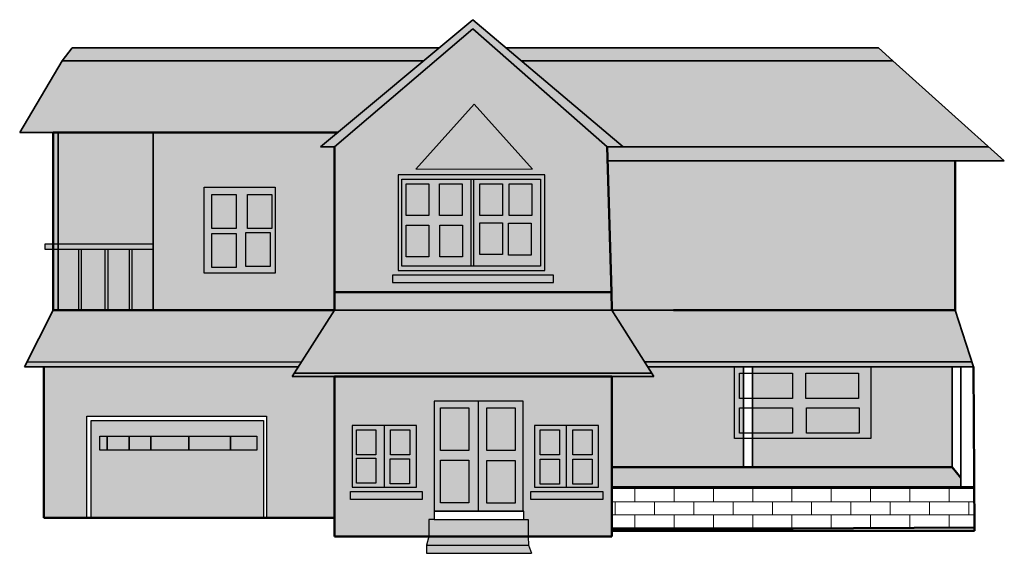
# Model space of a CAD drawing. Units: millimetres. Extents: x 69 to 5162, y 1088 to 3851.
import ezdxf

# ---------------------------------------------------------------- set-up
doc = ezdxf.new("R2010")
doc.units = ezdxf.units.MM
for name, color, linetype, lineweight in [('A-COLS', 7, 'Continuous', 35), ('A-DETL', 7, 'Continuous', 18), ('A-DOOR', 3, 'Continuous', 25), ('A-ELEV-PATT', 252, 'Continuous', 13), ('A-FLOR-HRAL', 6, 'Continuous', 25), ('A-FLOR-STRS', 3, 'Continuous', 25), ('A-GLAZ', 4, 'Continuous', 25), ('A-ROOF', 30, 'Continuous', 35), ('A-WALL', 7, 'Continuous', 50), ('A-WALL-PATT', 8, 'Continuous', 13)]:
    doc.layers.add(name, color=color, linetype=linetype, lineweight=lineweight)

msp = doc.modelspace()

# ---------------------------------------------------------------- hatches: boundary and pattern name
at = {"layer": 'A-ELEV-PATT'}
h = msp.add_hatch(color=256, dxfattribs=at)
h.set_gradient(color1=(169, 83, 160), color2=(169, 83, 160))
h.paths.add_polyline_path([(511.8, 2661), (389.1, 2661), (389.1, 2346.9), (511.8, 2346.9)])
h.paths.add_polyline_path([(636.7, 2661), (527.2, 2661), (527.2, 2346.9), (636.7, 2346.9)])
h.paths.add_polyline_path([(759.8, 2661), (651, 2661), (651, 2346.9), (759.8, 2346.9)])
h.paths.add_polyline_path([(374.7, 2661), (267.5, 2661), (267.5, 2346.9), (374.7, 2346.9)])
h.paths.add_polyline_path([(4892.2, 1533.1), (3131.8, 1533.1), (3131.8, 1431.2), (4937.5, 1431.2), (4937.5, 1478.9)])
h.paths.add_polyline_path([(944.6, 1695.1), (747.8, 1695.1), (747.8, 1621.5), (944.6, 1621.5)])
h.paths.add_polyline_path([(1159.7, 1695.1), (944.6, 1695.1), (944.6, 1621.5), (1159.7, 1621.5)])
h.paths.add_polyline_path([(1295.8, 1695.1), (1159.7, 1695.1), (1159.7, 1621.5), (1295.8, 1621.5)])
h.paths.add_polyline_path([(636.1, 1695.1), (521.5, 1695.1), (521.5, 1621.5), (636.1, 1621.5)])
h.paths.add_polyline_path([(747.8, 1695.1), (636.1, 1695.1), (636.1, 1621.5), (747.8, 1621.5)])
h.paths.add_polyline_path([(521.5, 1695.1), (482.9, 1695.1), (482.9, 1621.5), (521.5, 1621.5)])
h.paths.add_polyline_path([(2829.8, 2527.8), (1997.6, 2527.8), (1997.6, 2490.3), (2829.8, 2490.3)])
h.paths.add_polyline_path([(2786.1, 3048.5), (2027.1, 3048.5), (2027.1, 2552.8), (2786.1, 2552.8)])
h.paths.add_polyline_path([(2045.2, 2575.6), (2045.2, 3025.8), (2762.5, 3025.8), (2762.5, 2575.6)], flags=16)
h.paths.add_polyline_path([(2242.5, 2623.4), (2242.5, 2787.9), (2359.8, 2787.9), (2359.8, 2623.4)], flags=0)
h.paths.add_polyline_path([(2449.3, 2634.7), (2449.3, 2799.2), (2566.6, 2799.2), (2566.6, 2634.7)], flags=0)
h.paths.add_polyline_path([(2186, 2623.4), (2068.8, 2623.4), (2068.8, 2787.9), (2186, 2787.9)], flags=0)
h.paths.add_polyline_path([(2240.2, 2837.1), (2240.2, 3001.6), (2357.5, 3001.6), (2357.5, 2837.1)], flags=0)
h.paths.add_polyline_path([(2597.1, 2632.5), (2597.1, 2797), (2714.3, 2797), (2714.3, 2632.5)], flags=0)
h.paths.add_polyline_path([(2449.3, 2837.1), (2449.3, 3001.6), (2566.6, 3001.6), (2566.6, 2837.1)], flags=0)
h.paths.add_polyline_path([(2186, 2837.1), (2068.8, 2837.1), (2068.8, 3001.6), (2186, 3001.6)], flags=0)
h.paths.add_polyline_path([(2601.6, 2837.1), (2601.6, 3001.6), (2718.9, 3001.6), (2718.9, 2837.1)], flags=0)
h.paths.add_polyline_path([(1390.1, 2983.9), (1023.5, 2983.9), (1023.5, 2539.3), (1390.1, 2539.3)])
h.paths.add_polyline_path([(1239.1, 2749.6), (1365.2, 2749.6), (1365.2, 2573.5), (1239.1, 2573.5)], flags=16)
h.paths.add_polyline_path([(1189, 2568.7), (1062.9, 2568.7), (1062.9, 2744.7), (1189, 2744.7)], flags=16)
h.paths.add_polyline_path([(1247.2, 2769), (1247.2, 2945.1), (1373.3, 2945.1), (1373.3, 2769)], flags=16)
h.paths.add_polyline_path([(1189, 2769), (1062.9, 2769), (1062.9, 2945.1), (1189, 2945.1)], flags=16)
h.paths.add_polyline_path([(4471.7, 2052.7), (3859.7, 2052.7), (3859.7, 2020.4), (4066.3, 2020.4), (4066.3, 1889), (3859.7, 1889), (3859.7, 1841.9), (4066.3, 1841.9), (4066.3, 1710.5), (3859.7, 1710.5), (3859.7, 1683), (4471.7, 1683)])
h.paths.add_polyline_path([(4135.3, 1889), (4135.3, 2020.4), (4408.2, 2020.4), (4408.2, 1889)], flags=16)
h.paths.add_polyline_path([(4138.6, 1841.9), (4411.5, 1841.9), (4411.5, 1710.5), (4138.6, 1710.5)], flags=16)
h.paths.add_polyline_path([(3793.4, 1841.9), (3813.9, 1841.9), (3813.9, 1889), (3793.4, 1889), (3793.4, 2020.4), (3813.9, 2020.4), (3813.9, 2052.7), (3766.7, 2052.7), (3766.7, 1683), (3813.9, 1683), (3813.9, 1710.5), (3793.4, 1710.5)])
h.paths.add_polyline_path([(2442.6, 1875.6), (2212.5, 1875.6), (2212.5, 1306.4), (2442.6, 1306.4)])
h.paths.add_polyline_path([(2392.3, 1620), (2245.7, 1620), (2245.7, 1841.2), (2392.3, 1841.2)], flags=16)
h.paths.add_polyline_path([(2392.3, 1570.2), (2392.3, 1348.9), (2245.7, 1348.9), (2245.7, 1570.2)], flags=16)
h.paths.add_polyline_path([(2672.8, 1875.6), (2442.6, 1875.6), (2442.6, 1306.4), (2672.8, 1306.4)])
h.paths.add_polyline_path([(2486.1, 1620), (2486.1, 1841.2), (2632.7, 1841.2), (2632.7, 1620)], flags=16)
h.paths.add_polyline_path([(2486.1, 1568.7), (2632.7, 1568.7), (2632.7, 1347.5), (2486.1, 1347.5)], flags=16)
h.paths.add_polyline_path([(1955.6, 1749.4), (1789.6, 1749.4), (1789.6, 1431), (1955.6, 1431)])
h.paths.add_polyline_path([(1911.6, 1451.2), (1811.8, 1451.2), (1811.8, 1580.1), (1911.6, 1580.1)], flags=16)
h.paths.add_polyline_path([(1911.6, 1597.9), (1811.8, 1597.9), (1811.8, 1726.8), (1911.6, 1726.8)], flags=16)
h.paths.add_polyline_path([(2121.7, 1749.4), (1955.6, 1749.4), (1955.6, 1431), (2121.7, 1431)])
h.paths.add_polyline_path([(1986, 1577.2), (2085.8, 1577.2), (2085.8, 1448.3), (1986, 1448.3)], flags=16)
h.paths.add_polyline_path([(1986.9, 1597.9), (1986.9, 1726.8), (2086.7, 1726.8), (2086.7, 1597.9)], flags=16)
h.paths.add_polyline_path([(2151.4, 1408), (1779.5, 1408), (1779.5, 1367.3), (2151.4, 1367.3)])
h.paths.add_polyline_path([(3085.7, 1408), (2713.8, 1408), (2713.8, 1367.3), (3085.7, 1367.3)])
h.paths.add_polyline_path([(2897.4, 1749.4), (2731.3, 1749.4), (2731.3, 1431), (2897.4, 1431)])
h.paths.add_polyline_path([(2860.7, 1446.6), (2760.9, 1446.6), (2760.9, 1575.5), (2860.7, 1575.5)], flags=16)
h.paths.add_polyline_path([(2860.7, 1597.9), (2760.9, 1597.9), (2760.9, 1726.8), (2860.7, 1726.8)], flags=16)
h.paths.add_polyline_path([(3063.5, 1749.4), (2897.4, 1749.4), (2897.4, 1431), (3063.5, 1431)])
h.paths.add_polyline_path([(2929.9, 1575.5), (3029.7, 1575.5), (3029.7, 1446.6), (2929.9, 1446.6)], flags=16)
h.paths.add_polyline_path([(2929.9, 1597.9), (2929.9, 1726.8), (3029.7, 1726.8), (3029.7, 1597.9)], flags=16)
h.paths.add_polyline_path([(2238.2, 3704.6), (340.3, 3704.6), (288.6, 3637.4), (2157.7, 3637.4)])
h.paths.add_polyline_path([(4510.8, 3704.6), (2586.9, 3704.6), (2666.3, 3637.4), (4585.6, 3637.4)])
h.paths.add_polyline_path([(5080.6, 3193.1), (3107.7, 3193.1), (3109.9, 3119.6), (5162.5, 3119.6)])
h.paths.add_polyline_path([(2413.6, 3851.2), (1625.7, 3193.1), (1697.3, 3193.1), (2413.6, 3803.4), (3023.6, 3267.2), (3107.7, 3193.1), (3191.6, 3193.1)])
h.paths.add_polyline_path([(3129.9, 2440.9), (1697.3, 2440.9), (1697.3, 2346.9), (3131.8, 2346.9)])
h = msp.add_hatch(color=256, dxfattribs=at)
h.set_gradient(color1=(122, 175, 223), color2=(122, 175, 223))
h.paths.add_polyline_path([(1697.3, 3193.1), (1625.7, 3193.1), (1714.3, 3267.2), (759.8, 3267.2), (759.8, 2346.9), (1697.3, 2346.9), (1697.3, 2440.9)])
h.paths.add_polyline_path([(1023.5, 2983.9), (1390.1, 2983.9), (1390.1, 2539.3), (1023.5, 2539.3)], flags=16)
h.paths.add_polyline_path([(1062.9, 2945.1), (1189, 2945.1), (1189, 2769), (1062.9, 2769)], flags=0)
h.paths.add_polyline_path([(1062.9, 2744.7), (1189, 2744.7), (1189, 2568.7), (1062.9, 2568.7)], flags=0)
h.paths.add_polyline_path([(1247.2, 2945.1), (1373.3, 2945.1), (1373.3, 2769), (1247.2, 2769)], flags=0)
h.paths.add_polyline_path([(1239.1, 2749.6), (1365.2, 2749.6), (1365.2, 2573.5), (1239.1, 2573.5)], flags=0)
h.paths.add_polyline_path([(4907.8, 3119.6), (3109.9, 3119.6), (3129.9, 2440.9), (3131.8, 2346.9), (3452, 2346.9), (4907.8, 2346.9)])
h.paths.add_polyline_path([(3109.9, 3119.6), (3107.7, 3193.1), (3023.6, 3267.2), (2413.6, 3803.4), (1697.3, 3193.1), (1697.3, 2440.9), (3129.9, 2440.9)])
h.paths.add_polyline_path([(2786.1, 2552.8), (2027.1, 2552.8), (2027.1, 3048.5), (2786.1, 3048.5)], flags=16)
h.paths.add_polyline_path([(2762.5, 2575.6), (2045.2, 2575.6), (2045.2, 3025.8), (2762.5, 3025.8)], flags=0)
h.paths.add_polyline_path([(2718.9, 2837.1), (2601.6, 2837.1), (2601.6, 3001.6), (2718.9, 3001.6)], flags=0)
h.paths.add_polyline_path([(2714.3, 2797), (2714.3, 2632.5), (2597.1, 2632.5), (2597.1, 2797)], flags=0)
h.paths.add_polyline_path([(2722, 3077.5), (2119, 3077.5), (2420.5, 3413.6)], flags=16)
h.paths.add_polyline_path([(2829.8, 2527.8), (2829.8, 2490.3), (1997.6, 2490.3), (1997.6, 2527.8)], flags=16)
h.paths.add_polyline_path([(2566.6, 2837.1), (2449.3, 2837.1), (2449.3, 3001.6), (2566.6, 3001.6)], flags=0)
h.paths.add_polyline_path([(2566.6, 2799.2), (2566.6, 2634.7), (2449.3, 2634.7), (2449.3, 2799.2)], flags=0)
h.paths.add_polyline_path([(2357.5, 2837.1), (2240.2, 2837.1), (2240.2, 3001.6), (2357.5, 3001.6)], flags=0)
h.paths.add_polyline_path([(2359.8, 2787.9), (2359.8, 2623.4), (2242.5, 2623.4), (2242.5, 2787.9)], flags=0)
h.paths.add_polyline_path([(2186, 2837.1), (2068.8, 2837.1), (2068.8, 3001.6), (2186, 3001.6)], flags=0)
h.paths.add_polyline_path([(2186, 2787.9), (2186, 2623.4), (2068.8, 2623.4), (2068.8, 2787.9)], flags=0)
h.paths.add_polyline_path([(3766.7, 2052.7), (3318.2, 2052.7), (3349.6, 2003.2), (3131.8, 2003.2), (3131.8, 1533.1), (3813.9, 1533.1), (3813.9, 1683), (3766.7, 1683)])
h.paths.add_polyline_path([(4892.2, 2052.7), (4471.7, 2052.7), (4471.7, 1683), (3859.7, 1683), (3859.7, 1533.1), (4892.2, 1533.1)])
h.paths.add_polyline_path([(1697.3, 2003.2), (1478.5, 2003.2), (1510, 2052.7), (194.2, 2052.7), (194.2, 1271.1), (416.8, 1271.1), (416.8, 1797.4), (1345.9, 1797.4), (1345.9, 1271.1), (1697.3, 1271.1)])
h = msp.add_hatch(color=256, dxfattribs=at)
h.set_gradient(color1=(242, 103, 34), color2=(242, 103, 34))
h.paths.add_polyline_path([(2157.7, 3637.4), (288.6, 3637.4), (69, 3267.2), (242.5, 3267.2), (1714.3, 3267.2)])
h.paths.add_polyline_path([(4585.6, 3637.4), (2666.3, 3637.4), (3191.6, 3193.1), (5080.6, 3193.1)])
h.paths.add_polyline_path([(4907.8, 2346.9), (3452, 2346.9), (3131.8, 2346.9), (3300.9, 2080), (4995, 2080)])
h.paths.add_polyline_path([(1697.3, 2346.9), (242.5, 2346.9), (106.8, 2077.5), (1527.5, 2080)])
h.paths.add_polyline_path([(3131.8, 2346.9), (1697.3, 2346.9), (1527.5, 2080), (1489.6, 2020.5), (3338.6, 2020.5)])
h = msp.add_hatch(color=256, dxfattribs=at)
h.set_gradient(color1=(99, 100, 102), color2=(99, 100, 102))
h.paths.add_polyline_path([(759.8, 2690.2), (759.8, 3267.2), (267.5, 3267.2), (267.5, 2690.2)])
h.paths.add_polyline_path([(1330.1, 1271.1), (1330.1, 1775), (439.3, 1775), (439.3, 1271.1)])
h.paths.add_polyline_path([(482.9, 1621.5), (482.9, 1695.1), (1295.8, 1695.1), (1295.8, 1621.5)], flags=16)
h.paths.add_polyline_path([(2119, 3077.5), (2722, 3077.5), (2420.5, 3413.6)])
h.paths.add_polyline_path([(1697.3, 2003.2), (1697.3, 1175.3), (2185.2, 1175.3), (2185.2, 1262.3), (2212.5, 1262.3), (2212.5, 1306.4), (2212.5, 1875.6), (2672.8, 1875.6), (2672.8, 1306.4), (2677.5, 1306.4), (2677.5, 1262.3), (2699, 1262.3), (2699, 1175.3), (3131.8, 1175.3), (3131.8, 2003.2)])
h.paths.add_polyline_path([(3063.5, 1749.4), (3063.5, 1431), (2731.3, 1431), (2731.3, 1749.4)], flags=16)
h.paths.add_polyline_path([(2760.9, 1726.8), (2860.7, 1726.8), (2860.7, 1597.9), (2760.9, 1597.9)], flags=0)
h.paths.add_polyline_path([(2929.9, 1726.8), (3029.7, 1726.8), (3029.7, 1597.9), (2929.9, 1597.9)], flags=0)
h.paths.add_polyline_path([(2760.9, 1575.5), (2860.7, 1575.5), (2860.7, 1446.6), (2760.9, 1446.6)], flags=0)
h.paths.add_polyline_path([(2929.9, 1575.5), (3029.7, 1575.5), (3029.7, 1446.6), (2929.9, 1446.6)], flags=0)
h.paths.add_polyline_path([(3085.7, 1408), (3085.7, 1367.3), (2713.8, 1367.3), (2713.8, 1408)], flags=16)
h.paths.add_polyline_path([(2121.7, 1749.4), (2121.7, 1431), (1789.6, 1431), (1789.6, 1749.4)], flags=16)
h.paths.add_polyline_path([(2086.7, 1726.8), (2086.7, 1597.9), (1986.9, 1597.9), (1986.9, 1726.8)], flags=0)
h.paths.add_polyline_path([(2085.8, 1577.2), (2085.8, 1448.3), (1986, 1448.3), (1986, 1577.2)], flags=0)
h.paths.add_polyline_path([(2151.4, 1408), (2151.4, 1367.3), (1779.5, 1367.3), (1779.5, 1408)], flags=16)
h.paths.add_polyline_path([(1911.6, 1726.8), (1911.6, 1597.9), (1811.8, 1597.9), (1811.8, 1726.8)], flags=0)
h.paths.add_polyline_path([(1911.6, 1580.1), (1911.6, 1451.2), (1811.8, 1451.2), (1811.8, 1580.1)], flags=0)
h = msp.add_hatch(color=256, dxfattribs=at)
h.set_gradient(color1=(255, 255, 255))
h.paths.add_polyline_path([(267.5, 3267.2), (242.5, 3267.2), (242.5, 2690.2), (267.5, 2690.2)])
h.paths.add_polyline_path([(759.8, 2690.2), (267.5, 2690.2), (267.5, 2661), (759.8, 2661)])
h.paths.add_polyline_path([(651, 2661), (636.7, 2661), (636.7, 2346.9), (651, 2346.9)])
h.paths.add_polyline_path([(267.5, 2661), (242.5, 2661), (242.5, 2346.9), (267.5, 2346.9)])
h.paths.add_polyline_path([(267.5, 2690.2), (242.5, 2690.2), (242.5, 2661), (267.5, 2661)])
h.paths.add_polyline_path([(242.5, 2690.2), (200.1, 2690.2), (200.1, 2661), (242.5, 2661)])
h.paths.add_polyline_path([(389.1, 2661), (374.7, 2661), (374.7, 2346.9), (389.1, 2346.9)])
h.paths.add_polyline_path([(527.2, 2661), (511.8, 2661), (511.8, 2346.9), (527.2, 2346.9)])
h.paths.add_polyline_path([(1527.5, 2080), (106.8, 2077.5), (94.3, 2052.7), (1510, 2052.7)])
h.paths.add_polyline_path([(3338.6, 2020.5), (1489.6, 2020.5), (1478.5, 2003.2), (1697.3, 2003.2), (3131.8, 2003.2), (3349.6, 2003.2)])
h.paths.add_polyline_path([(4995, 2080), (3300.9, 2080), (3318.2, 2052.7), (5003.9, 2052.7)])
h = msp.add_hatch(color=256, dxfattribs=at)
h.set_gradient(color1=(0, 255, 255), color2=(0, 255, 255))
h.paths.add_polyline_path([(2068.8, 2837.1), (2186, 2837.1), (2186, 3001.6), (2068.8, 3001.6)])
h.paths.add_polyline_path([(2240.2, 2837.1), (2357.5, 2837.1), (2357.5, 3001.6), (2240.2, 3001.6)])
h.paths.add_polyline_path([(2242.5, 2787.9), (2242.5, 2623.4), (2359.8, 2623.4), (2359.8, 2787.9)])
h.paths.add_polyline_path([(2186, 2787.9), (2068.8, 2787.9), (2068.8, 2623.4), (2186, 2623.4)])
h.paths.add_polyline_path([(2449.3, 2837.1), (2566.6, 2837.1), (2566.6, 3001.6), (2449.3, 3001.6)])
h.paths.add_polyline_path([(2601.6, 2837.1), (2718.9, 2837.1), (2718.9, 3001.6), (2601.6, 3001.6)])
h.paths.add_polyline_path([(2714.3, 2797), (2597.1, 2797), (2597.1, 2632.5), (2714.3, 2632.5)])
h.paths.add_polyline_path([(2449.3, 2634.7), (2566.6, 2634.7), (2566.6, 2799.2), (2449.3, 2799.2)])
h.paths.add_polyline_path([(1247.2, 2769), (1373.3, 2769), (1373.3, 2945.1), (1247.2, 2945.1)])
h.paths.add_polyline_path([(1062.9, 2769), (1189, 2769), (1189, 2945.1), (1062.9, 2945.1)])
h.paths.add_polyline_path([(1062.9, 2568.7), (1189, 2568.7), (1189, 2744.7), (1062.9, 2744.7)])
h.paths.add_polyline_path([(1365.2, 2749.6), (1239.1, 2749.6), (1239.1, 2573.5), (1365.2, 2573.5)])
h.paths.add_polyline_path([(1811.8, 1597.9), (1911.6, 1597.9), (1911.6, 1726.8), (1811.8, 1726.8)])
h.paths.add_polyline_path([(2086.7, 1597.9), (2086.7, 1726.8), (1986.9, 1726.8), (1986.9, 1597.9)])
h.paths.add_polyline_path([(1986, 1448.3), (2085.8, 1448.3), (2085.8, 1577.2), (1986, 1577.2)])
h.paths.add_polyline_path([(1911.6, 1580.1), (1811.8, 1580.1), (1811.8, 1451.2), (1911.6, 1451.2)])
h.paths.add_polyline_path([(2392.3, 1841.2), (2245.7, 1841.2), (2245.7, 1620), (2392.3, 1620)])
h.paths.add_polyline_path([(2860.7, 1597.9), (2860.7, 1726.8), (2760.9, 1726.8), (2760.9, 1597.9)])
h.paths.add_polyline_path([(2860.7, 1575.5), (2760.9, 1575.5), (2760.9, 1446.6), (2860.7, 1446.6)])
h.paths.add_polyline_path([(3029.7, 1726.8), (2929.9, 1726.8), (2929.9, 1597.9), (3029.7, 1597.9)])
h.paths.add_polyline_path([(3029.7, 1575.5), (2929.9, 1575.5), (2929.9, 1446.6), (3029.7, 1446.6)])
h.paths.add_polyline_path([(4066.3, 1889), (4066.3, 2020.4), (3859.7, 2020.4), (3859.7, 1889)])
h.paths.add_polyline_path([(4408.2, 1889), (4408.2, 2020.4), (4135.3, 2020.4), (4135.3, 1889)])
h.paths.add_polyline_path([(4411.5, 1710.5), (4411.5, 1841.9), (4138.6, 1841.9), (4138.6, 1710.5)])
h.paths.add_polyline_path([(4066.3, 1710.5), (4066.3, 1841.9), (3859.7, 1841.9), (3859.7, 1710.5)])
h.paths.add_polyline_path([(3793.4, 1710.5), (3813.9, 1710.5), (3813.9, 1841.9), (3793.4, 1841.9)])
h.paths.add_polyline_path([(3813.9, 2020.4), (3793.4, 2020.4), (3793.4, 1889), (3813.9, 1889)])
h = msp.add_hatch(color=256, dxfattribs=at)
h.set_gradient(color1=(16, 86, 137), color2=(34, 52, 110))
h.paths.add_polyline_path([(2068.8, 2837.1), (2186, 2837.1), (2186, 3001.6), (2068.8, 3001.6)])
h.paths.add_polyline_path([(2240.2, 3001.6), (2240.2, 2837.1), (2357.5, 2837.1), (2357.5, 3001.6)])
h.paths.add_polyline_path([(2449.3, 3001.6), (2449.3, 2837.1), (2566.6, 2837.1), (2566.6, 3001.6)])
h.paths.add_polyline_path([(2601.6, 2837.1), (2718.9, 2837.1), (2718.9, 3001.6), (2601.6, 3001.6)])
h.paths.add_polyline_path([(2597.1, 2632.5), (2714.3, 2632.5), (2714.3, 2797), (2597.1, 2797)])
h.paths.add_polyline_path([(2449.3, 2634.7), (2566.6, 2634.7), (2566.6, 2799.2), (2449.3, 2799.2)])
h.paths.add_polyline_path([(2359.8, 2787.9), (2242.5, 2787.9), (2242.5, 2623.4), (2359.8, 2623.4)])
h.paths.add_polyline_path([(2068.8, 2787.9), (2068.8, 2623.4), (2186, 2623.4), (2186, 2787.9)])
h.paths.add_polyline_path([(1247.2, 2945.1), (1247.2, 2769), (1373.3, 2769), (1373.3, 2945.1)])
h.paths.add_polyline_path([(1365.2, 2749.6), (1239.1, 2749.6), (1239.1, 2573.5), (1365.2, 2573.5)])
h.paths.add_polyline_path([(1189, 2945.1), (1062.9, 2945.1), (1062.9, 2769), (1189, 2769)])
h.paths.add_polyline_path([(1062.9, 2744.7), (1062.9, 2568.7), (1189, 2568.7), (1189, 2744.7)])
h.paths.add_polyline_path([(1911.6, 1726.8), (1811.8, 1726.8), (1811.8, 1597.9), (1911.6, 1597.9)])
h.paths.add_polyline_path([(1911.6, 1580.1), (1811.8, 1580.1), (1811.8, 1451.2), (1911.6, 1451.2)])
h.paths.add_polyline_path([(1986.9, 1597.9), (2086.7, 1597.9), (2086.7, 1726.8), (1986.9, 1726.8)])
h.paths.add_polyline_path([(1986, 1448.3), (2085.8, 1448.3), (2085.8, 1577.2), (1986, 1577.2)])
h.paths.add_polyline_path([(2760.9, 1597.9), (2860.7, 1597.9), (2860.7, 1726.8), (2760.9, 1726.8)])
h.paths.add_polyline_path([(2929.9, 1597.9), (3029.7, 1597.9), (3029.7, 1726.8), (2929.9, 1726.8)])
h.paths.add_polyline_path([(2929.9, 1446.6), (3029.7, 1446.6), (3029.7, 1575.5), (2929.9, 1575.5)])
h.paths.add_polyline_path([(2760.9, 1575.5), (2760.9, 1446.6), (2860.7, 1446.6), (2860.7, 1575.5)])
h.paths.add_polyline_path([(4066.3, 1889), (4066.3, 2020.4), (3859.7, 2020.4), (3859.7, 1889)])
h.paths.add_polyline_path([(4408.2, 1889), (4408.2, 2020.4), (4135.3, 2020.4), (4135.3, 1889)])
h.paths.add_polyline_path([(4411.5, 1710.5), (4411.5, 1841.9), (4138.6, 1841.9), (4138.6, 1710.5)])
h.paths.add_polyline_path([(3859.7, 1841.9), (3859.7, 1710.5), (4066.3, 1710.5), (4066.3, 1841.9)])
h.paths.add_polyline_path([(3793.4, 1889), (3813.9, 1889), (3813.9, 2020.4), (3793.4, 2020.4)])
h.paths.add_polyline_path([(3793.4, 1710.5), (3813.9, 1710.5), (3813.9, 1841.9), (3793.4, 1841.9)])
h = msp.add_hatch(color=256, dxfattribs=at)
h.set_gradient(color1=(237, 31, 36), color2=(255, 0, 0))
h.paths.add_polyline_path([(2392.3, 1841.2), (2245.7, 1841.2), (2245.7, 1620), (2392.3, 1620)])
h.paths.add_polyline_path([(2632.7, 1620), (2632.7, 1841.2), (2486.1, 1841.2), (2486.1, 1620)])
h.paths.add_polyline_path([(2632.7, 1568.7), (2486.1, 1568.7), (2486.1, 1347.5), (2632.7, 1347.5)])
h.paths.add_polyline_path([(2392.3, 1570.2), (2245.7, 1570.2), (2245.7, 1348.9), (2392.3, 1348.9)])
h = msp.add_hatch(color=256, dxfattribs=at)
h.set_gradient(color1=(19, 103, 52), color2=(19, 103, 52))
h.paths.add_polyline_path([(2699, 1262.3), (2677.5, 1262.3), (2212.5, 1262.3), (2185.2, 1262.3), (2185.2, 1175.3), (2699, 1175.3)])
h.paths.add_polyline_path([(2699, 1175.3), (2185.2, 1175.3), (2174.2, 1129.6), (2700.8, 1129.6)])
h.paths.add_polyline_path([(2700.8, 1129.6), (2174.2, 1129.6), (2174.2, 1087.8), (2715.9, 1087.8)])
at = {"layer": 'A-WALL-PATT'}
h = msp.add_hatch(dxfattribs=at)
h.set_pattern_fill('AR-BRSTD', color=256)
h.paths.add_polyline_path([(5007.5, 1431.2), (3131.8, 1431.2), (3131.8, 1210.9), (5008.7, 1221.8)])

# ---------------------------------------------------------------- linework, layer by layer
at = {"layer": 'A-COLS'}
for p, q in [((267.5, 2346.9), (267.5, 3267.2)), ((759.8, 2346.9), (759.8, 3267.2)), ((3813.9, 1533.1), (3813.9, 2052.7)), ((3859.7, 1533.1), (3859.7, 2052.7)), ((4892.2, 1533.1), (4892.2, 2052.7)), ((4937.5, 1431.2), (4937.5, 2052.7))]:
    msp.add_line(p, q, dxfattribs=at)
at = {"layer": 'A-DETL'}
for p, q in [((2119, 3077.5), (2420.5, 3413.6)), ((2420.5, 3413.6), (2722, 3077.5)), ((2119, 3077.5), (2722, 3077.5))]:
    msp.add_line(p, q, dxfattribs=at)
at = {"layer": 'A-DOOR'}
for p, q in [((2442.6, 1306.4), (2442.6, 1875.6)), ((416.8, 1271.1), (416.8, 1797.4)), ((416.8, 1797.4), (1345.9, 1797.4)), ((1345.9, 1797.4), (1345.9, 1271.1)), ((439.3, 1271.1), (439.3, 1775)), ((439.3, 1775), (1330.1, 1775)), ((1330.1, 1775), (1330.1, 1271.1))]:
    msp.add_line(p, q, dxfattribs=at)
for points in [[(2212.5, 1306.4), (2672.8, 1306.4), (2672.8, 1875.6), (2212.5, 1875.6)], [(2245.7, 1841.2), (2392.3, 1841.2), (2392.3, 1620), (2245.7, 1620)], [(2486.1, 1841.2), (2632.7, 1841.2), (2632.7, 1620), (2486.1, 1620)], [(482.9, 1695.1), (1295.8, 1695.1), (1295.8, 1621.5), (482.9, 1621.5)], [(521.5, 1695.1), (521.5, 1695.1), (521.5, 1621.5), (521.5, 1621.5)], [(636.1, 1695.1), (636.1, 1695.1), (636.1, 1621.5), (636.1, 1621.5)], [(747.8, 1695.1), (747.8, 1695.1), (747.8, 1621.5), (747.8, 1621.5)], [(944.6, 1695.1), (944.6, 1695.1), (944.6, 1621.5), (944.6, 1621.5)], [(1159.7, 1695.1), (1159.7, 1695.1), (1159.7, 1621.5), (1159.7, 1621.5)], [(2245.7, 1570.2), (2392.3, 1570.2), (2392.3, 1348.9), (2245.7, 1348.9)], [(2486.1, 1568.7), (2632.7, 1568.7), (2632.7, 1347.5), (2486.1, 1347.5)], [(2212.5, 1262.3), (2677.5, 1262.3), (2677.5, 1306.4), (2212.5, 1306.4)]]:
    msp.add_lwpolyline(points, close=True, dxfattribs=at)
at = {"layer": 'A-FLOR-HRAL'}
for p, q in [((200.1, 2661), (200.1, 2690.2)), ((200.1, 2690.2), (759.8, 2690.2)), ((759.8, 2661), (200.1, 2661)), ((374.7, 2346.9), (374.7, 2661)), ((389.1, 2346.9), (389.1, 2661)), ((511.8, 2346.9), (511.8, 2661)), ((527.2, 2346.9), (527.2, 2661)), ((636.7, 2346.9), (636.7, 2661)), ((651, 2346.9), (651, 2661))]:
    msp.add_line(p, q, dxfattribs=at)
at = {"layer": 'A-FLOR-STRS'}
for p, q in [((2212.5, 1262.3), (2185.2, 1262.3)), ((2185.2, 1262.3), (2185.2, 1175.3)), ((2677.5, 1262.3), (2699, 1262.3)), ((2699, 1262.3), (2699, 1175.3)), ((2185.2, 1175.3), (2174.2, 1129.6)), ((2699, 1175.3), (2700.8, 1129.6)), ((2174.2, 1129.6), (2174.2, 1087.8)), ((2174.2, 1129.6), (2700.8, 1129.6)), ((2700.8, 1129.6), (2715.9, 1087.8)), ((2174.2, 1087.8), (2715.9, 1087.8))]:
    msp.add_line(p, q, dxfattribs=at)
at = {"layer": 'A-GLAZ'}
for p, q in [((2403.9, 2575.6), (2403.9, 3025.8)), ((2418, 2575.6), (2418, 3025.8)), ((1955.6, 1431), (1955.6, 1749.4)), ((2897.4, 1431), (2897.4, 1749.4))]:
    msp.add_line(p, q, dxfattribs=at)
for points in [[(2027.1, 2552.8), (2786.1, 2552.8), (2786.1, 3048.5), (2027.1, 3048.5)], [(2045.2, 3025.8), (2762.5, 3025.8), (2762.5, 2575.6), (2045.2, 2575.6)], [(1023.5, 2983.9), (1390.1, 2983.9), (1390.1, 2539.3), (1023.5, 2539.3)], [(2068.8, 3001.6), (2186, 3001.6), (2186, 2837.1), (2068.8, 2837.1)], [(2240.2, 3001.6), (2357.5, 3001.6), (2357.5, 2837.1), (2240.2, 2837.1)], [(2449.3, 3001.6), (2566.6, 3001.6), (2566.6, 2837.1), (2449.3, 2837.1)], [(2601.6, 3001.6), (2718.9, 3001.6), (2718.9, 2837.1), (2601.6, 2837.1)], [(1062.9, 2945.1), (1189, 2945.1), (1189, 2769), (1062.9, 2769)], [(1247.2, 2945.1), (1373.3, 2945.1), (1373.3, 2769), (1247.2, 2769)], [(2068.8, 2787.9), (2186, 2787.9), (2186, 2623.4), (2068.8, 2623.4)], [(2242.5, 2787.9), (2359.8, 2787.9), (2359.8, 2623.4), (2242.5, 2623.4)], [(2449.3, 2799.2), (2566.6, 2799.2), (2566.6, 2634.7), (2449.3, 2634.7)], [(2597.1, 2797), (2714.3, 2797), (2714.3, 2632.5), (2597.1, 2632.5)], [(1062.9, 2744.7), (1189, 2744.7), (1189, 2568.7), (1062.9, 2568.7)], [(1239.1, 2749.6), (1365.2, 2749.6), (1365.2, 2573.5), (1239.1, 2573.5)], [(1997.6, 2490.3), (2829.8, 2490.3), (2829.8, 2527.8), (1997.6, 2527.8)], [(3766.7, 2052.7), (4471.7, 2052.7), (4471.7, 1683), (3766.7, 1683)], [(3793.4, 2020.4), (4066.3, 2020.4), (4066.3, 1889), (3793.4, 1889)], [(4135.3, 2020.4), (4408.2, 2020.4), (4408.2, 1889), (4135.3, 1889)], [(3793.4, 1841.9), (4066.3, 1841.9), (4066.3, 1710.5), (3793.4, 1710.5)], [(4138.6, 1841.9), (4411.5, 1841.9), (4411.5, 1710.5), (4138.6, 1710.5)], [(1789.6, 1431), (2121.7, 1431), (2121.7, 1749.4), (1789.6, 1749.4)], [(2731.3, 1431), (3063.5, 1431), (3063.5, 1749.4), (2731.3, 1749.4)], [(1811.8, 1726.8), (1911.6, 1726.8), (1911.6, 1597.9), (1811.8, 1597.9)], [(1986.9, 1726.8), (2086.7, 1726.8), (2086.7, 1597.9), (1986.9, 1597.9)], [(2760.9, 1726.8), (2860.7, 1726.8), (2860.7, 1597.9), (2760.9, 1597.9)], [(2929.9, 1726.8), (3029.7, 1726.8), (3029.7, 1597.9), (2929.9, 1597.9)], [(1811.8, 1580.1), (1911.6, 1580.1), (1911.6, 1451.2), (1811.8, 1451.2)], [(1986, 1577.2), (2085.8, 1577.2), (2085.8, 1448.3), (1986, 1448.3)], [(2760.9, 1575.5), (2860.7, 1575.5), (2860.7, 1446.6), (2760.9, 1446.6)], [(2929.9, 1575.5), (3029.7, 1575.5), (3029.7, 1446.6), (2929.9, 1446.6)], [(1779.5, 1408), (2151.4, 1408), (2151.4, 1367.3), (1779.5, 1367.3)], [(2713.8, 1408), (3085.7, 1408), (3085.7, 1367.3), (2713.8, 1367.3)]]:
    msp.add_lwpolyline(points, close=True, dxfattribs=at)
at = {"layer": 'A-ROOF'}
for p, q in [((1625.7, 3193.1), (2413.6, 3851.2)), ((2413.6, 3851.2), (3191.6, 3193.1)), ((1697.3, 3193.1), (2413.6, 3803.4)), ((2413.6, 3803.4), (3023.6, 3267.2)), ((288.6, 3637.4), (340.3, 3704.6)), ((340.3, 3704.6), (2238.2, 3704.6)), ((2586.9, 3704.6), (4510.8, 3704.6)), ((4585.6, 3637.4), (4510.8, 3704.6)), ((69, 3267.2), (288.6, 3637.4)), ((288.6, 3637.4), (2157.7, 3637.4)), ((2666.3, 3637.4), (4585.6, 3637.4)), ((5162.5, 3119.6), (4585.6, 3637.4)), ((242.5, 3267.2), (69, 3267.2)), ((3023.6, 3267.2), (3107.7, 3193.1)), ((1697.3, 3193.1), (1625.7, 3193.1)), ((3107.7, 3193.1), (3191.6, 3193.1)), ((3107.7, 3193.1), (5080.6, 3193.1)), ((3109.9, 3119.6), (5162.5, 3119.6)), ((242.5, 2346.9), (94.3, 2052.7)), ((1478.5, 2003.2), (1697.3, 2346.9)), ((1697.3, 2346.9), (3452, 2346.9)), ((3349.6, 2003.2), (3131.8, 2346.9)), ((4907.8, 2346.9), (5003.9, 2052.7)), ((1510, 2052.7), (94.3, 2052.7)), ((106.8, 2077.5), (1527.5, 2080)), ((3300.9, 2080), (4995, 2080)), ((3318.2, 2052.7), (5003.9, 2052.7)), ((1697.3, 2003.2), (1478.5, 2003.2)), ((1489.6, 2020.5), (3338.6, 2020.5)), ((3131.8, 2003.2), (3349.6, 2003.2))]:
    msp.add_line(p, q, dxfattribs=at)
at = {"layer": 'A-WALL'}
for p, q in [((242.5, 2346.9), (242.5, 3267.2)), ((242.5, 3267.2), (1714.3, 3267.2)), ((1697.3, 2440.9), (1697.3, 3193.1)), ((3107.7, 3193.1), (3129.9, 2440.9)), ((4907.8, 2346.9), (4907.8, 3119.6)), ((1697.3, 2346.9), (1697.3, 2440.9)), ((3129.9, 2440.9), (3131.8, 2346.9)), ((1697.3, 2346.9), (242.5, 2346.9)), ((3452, 2346.9), (4907.8, 2346.9)), ((194.2, 1271.1), (194.2, 2052.7)), ((5008.8, 1203.4), (5003.9, 2052.7)), ((1697.3, 1175.3), (1697.3, 2003.2)), ((1697.3, 2003.2), (3131.8, 2003.2)), ((3131.8, 1175.3), (3131.8, 2003.2)), ((4892.2, 1533.1), (3131.8, 1533.1)), ((4892.2, 1533.1), (4937.5, 1478.9)), ((3131.8, 1431.2), (5007.5, 1431.2)), ((1697.3, 1271.1), (194.2, 1271.1)), ((1697.3, 1175.3), (3131.8, 1175.3)), ((3131.8, 1210.9), (5008.7, 1221.8)), ((3131.8, 1203.4), (5008.8, 1203.4))]:
    msp.add_line(p, q, dxfattribs=at)
msp.add_lwpolyline([(1697.3, 2440.9), (3129.9, 2440.9)], dxfattribs=at)

doc.saveas('drawing.dxf')
